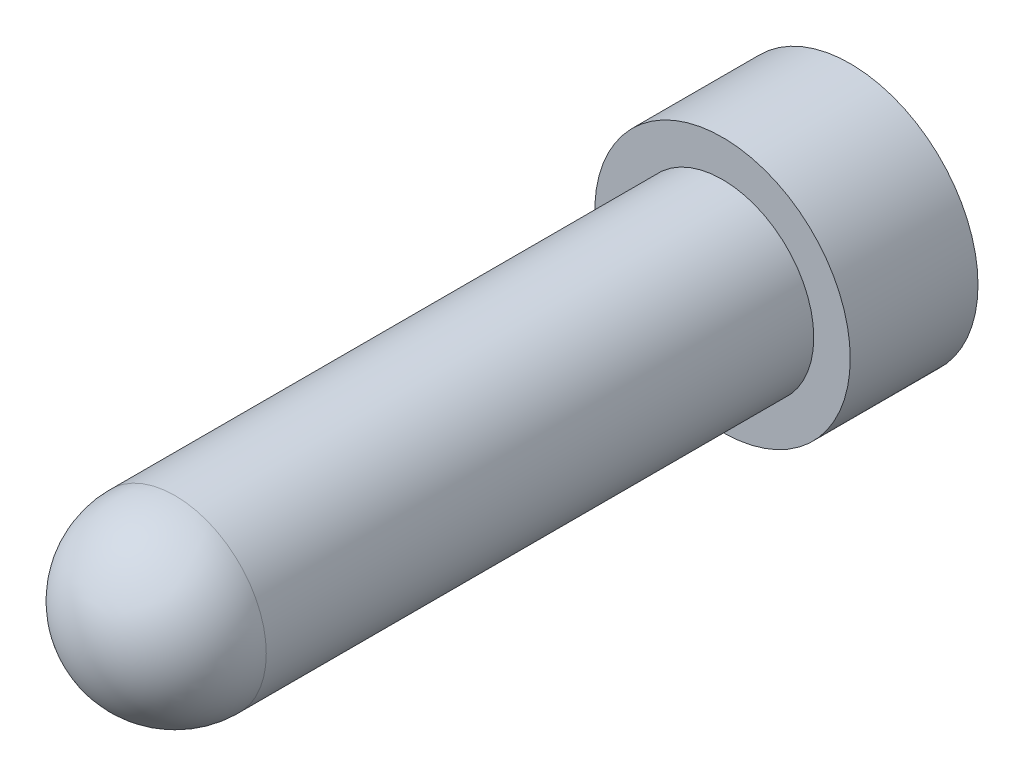
ISO-10303-21;
HEADER;
FILE_DESCRIPTION(('STEP AP214'),'2;1');
FILE_NAME('part.step','',(''),(''),'','','');
FILE_SCHEMA(('AUTOMOTIVE_DESIGN { 1 0 10303 214 1 1 1 1 }'));
ENDSEC;
DATA;
#1=APPLICATION_CONTEXT('core data for automotive mechanical design processes');
#2=APPLICATION_PROTOCOL_DEFINITION('international standard','automotive_design',2000,#1);
#3=PRODUCT_CONTEXT('',#1,'mechanical');
#4=PRODUCT('Part','Part','',(#3));
#5=PRODUCT_RELATED_PRODUCT_CATEGORY('part','',(#4));
#6=PRODUCT_DEFINITION_FORMATION('','',#4);
#7=PRODUCT_DEFINITION_CONTEXT('part definition',#1,'design');
#8=PRODUCT_DEFINITION('design','',#6,#7);
#9=PRODUCT_DEFINITION_SHAPE('','',#8);
#10=(LENGTH_UNIT() NAMED_UNIT(*) SI_UNIT(.MILLI.,.METRE.));
#11=(NAMED_UNIT(*) PLANE_ANGLE_UNIT() SI_UNIT($,.RADIAN.));
#12=(NAMED_UNIT(*) SI_UNIT($,.STERADIAN.) SOLID_ANGLE_UNIT());
#13=UNCERTAINTY_MEASURE_WITH_UNIT(LENGTH_MEASURE(1.E-05),#10,'distance_accuracy_value','');
#14=(GEOMETRIC_REPRESENTATION_CONTEXT(3) GLOBAL_UNCERTAINTY_ASSIGNED_CONTEXT((#13)) GLOBAL_UNIT_ASSIGNED_CONTEXT((#10,
#11,#12)) REPRESENTATION_CONTEXT('',''));
#15=CARTESIAN_POINT('',(0.,0.,0.));
#16=DIRECTION('',(0.,0.,1.));
#17=DIRECTION('',(1.,0.,0.));
#18=AXIS2_PLACEMENT_3D('',#15,#16,#17);
#19=CARTESIAN_POINT('',(0.,0.,7.));
#20=DIRECTION('',(0.,0.,-1.));
#21=DIRECTION('',(-1.,0.,0.));
#22=AXIS2_PLACEMENT_3D('',#19,#20,#21);
#23=CYLINDRICAL_SURFACE('',#22,7.);
#24=CARTESIAN_POINT('',(0.,0.,7.));
#25=DIRECTION('',(0.,0.,1.));
#26=DIRECTION('',(1.,0.,0.));
#27=AXIS2_PLACEMENT_3D('',#24,#25,#26);
#28=CIRCLE('',#27,7.);
#29=CARTESIAN_POINT('',(7.,0.,7.));
#30=VERTEX_POINT('',#29);
#31=EDGE_CURVE('E149',#30,#30,#28,.T.);
#32=ORIENTED_EDGE('',*,*,#31,.F.);
#33=EDGE_LOOP('',(#32));
#34=FACE_BOUND('',#33,.T.);
#35=CARTESIAN_POINT('',(0.,0.,0.));
#36=DIRECTION('',(0.,0.,1.));
#37=DIRECTION('',(1.,0.,0.));
#38=AXIS2_PLACEMENT_3D('',#35,#36,#37);
#39=CIRCLE('',#38,7.);
#40=CARTESIAN_POINT('',(7.,0.,0.));
#41=VERTEX_POINT('',#40);
#42=EDGE_CURVE('E143',#41,#41,#39,.T.);
#43=ORIENTED_EDGE('',*,*,#42,.T.);
#44=EDGE_LOOP('',(#43));
#45=FACE_BOUND('',#44,.T.);
#46=ADVANCED_FACE('F39',(#34,#45),#23,.T.);
#47=CARTESIAN_POINT('',(0.,0.,7.));
#48=DIRECTION('',(0.,0.,1.));
#49=DIRECTION('',(1.,0.,0.));
#50=AXIS2_PLACEMENT_3D('',#47,#48,#49);
#51=PLANE('',#50);
#52=CARTESIAN_POINT('',(0.,0.,7.));
#53=DIRECTION('',(0.,0.,1.));
#54=DIRECTION('',(1.,0.,0.));
#55=AXIS2_PLACEMENT_3D('',#52,#53,#54);
#56=CIRCLE('',#55,5.);
#57=CARTESIAN_POINT('',(5.,0.,7.));
#58=VERTEX_POINT('',#57);
#59=EDGE_CURVE('E50',#58,#58,#56,.T.);
#60=ORIENTED_EDGE('',*,*,#59,.F.);
#61=EDGE_LOOP('',(#60));
#62=FACE_BOUND('',#61,.T.);
#63=ORIENTED_EDGE('',*,*,#31,.T.);
#64=EDGE_LOOP('',(#63));
#65=FACE_BOUND('',#64,.T.);
#66=ADVANCED_FACE('F158',(#62,#65),#51,.T.);
#67=CARTESIAN_POINT('',(0.,0.,0.));
#68=DIRECTION('',(0.,0.,1.));
#69=DIRECTION('',(1.,0.,0.));
#70=AXIS2_PLACEMENT_3D('',#67,#68,#69);
#71=PLANE('',#70);
#72=DIRECTION('',(0.5,0.866025403784439,0.));
#73=VECTOR('',#72,1.);
#74=CARTESIAN_POINT('',(-5.77350269189626,0.,0.));
#75=LINE('',#74,#73);
#76=CARTESIAN_POINT('',(-5.77350269189626,0.,0.));
#77=VERTEX_POINT('',#76);
#78=CARTESIAN_POINT('',(-2.88675134594813,5.,0.));
#79=VERTEX_POINT('',#78);
#80=EDGE_CURVE('E126',#77,#79,#75,.T.);
#81=ORIENTED_EDGE('',*,*,#80,.F.);
#82=DIRECTION('',(-0.5,0.866025403784439,0.));
#83=VECTOR('',#82,1.);
#84=CARTESIAN_POINT('',(-2.88675134594813,-5.,0.));
#85=LINE('',#84,#83);
#86=CARTESIAN_POINT('',(-2.88675134594813,-5.,0.));
#87=VERTEX_POINT('',#86);
#88=EDGE_CURVE('E53',#87,#77,#85,.T.);
#89=ORIENTED_EDGE('',*,*,#88,.F.);
#90=DIRECTION('',(-1.,0.,0.));
#91=VECTOR('',#90,1.);
#92=CARTESIAN_POINT('',(2.88675134594813,-5.,0.));
#93=LINE('',#92,#91);
#94=CARTESIAN_POINT('',(2.88675134594813,-5.,0.));
#95=VERTEX_POINT('',#94);
#96=EDGE_CURVE('E140',#95,#87,#93,.T.);
#97=ORIENTED_EDGE('',*,*,#96,.F.);
#98=DIRECTION('',(-0.5,-0.866025403784439,0.));
#99=VECTOR('',#98,1.);
#100=CARTESIAN_POINT('',(5.77350269189626,0.,0.));
#101=LINE('',#100,#99);
#102=CARTESIAN_POINT('',(5.77350269189626,0.,0.));
#103=VERTEX_POINT('',#102);
#104=EDGE_CURVE('E132',#103,#95,#101,.T.);
#105=ORIENTED_EDGE('',*,*,#104,.F.);
#106=DIRECTION('',(0.5,-0.866025403784439,0.));
#107=VECTOR('',#106,1.);
#108=CARTESIAN_POINT('',(2.88675134594813,5.,0.));
#109=LINE('',#108,#107);
#110=CARTESIAN_POINT('',(2.88675134594813,5.,0.));
#111=VERTEX_POINT('',#110);
#112=EDGE_CURVE('E105',#111,#103,#109,.T.);
#113=ORIENTED_EDGE('',*,*,#112,.F.);
#114=DIRECTION('',(1.,0.,0.));
#115=VECTOR('',#114,1.);
#116=CARTESIAN_POINT('',(-2.88675134594813,5.,0.));
#117=LINE('',#116,#115);
#118=EDGE_CURVE('E133',#79,#111,#117,.T.);
#119=ORIENTED_EDGE('',*,*,#118,.F.);
#120=EDGE_LOOP('',(#81,#89,#97,#105,#113,#119));
#121=FACE_BOUND('',#120,.T.);
#122=ORIENTED_EDGE('',*,*,#42,.F.);
#123=EDGE_LOOP('',(#122));
#124=FACE_BOUND('',#123,.T.);
#125=ADVANCED_FACE('F154',(#121,#124),#71,.F.);
#126=CARTESIAN_POINT('',(0.,0.,42.));
#127=DIRECTION('',(0.,0.,-1.));
#128=DIRECTION('',(-1.,0.,0.));
#129=AXIS2_PLACEMENT_3D('',#126,#127,#128);
#130=CYLINDRICAL_SURFACE('',#129,5.);
#131=CARTESIAN_POINT('',(0.,0.,37.));
#132=DIRECTION('',(0.,0.,-1.));
#133=DIRECTION('',(-1.,0.,0.));
#134=AXIS2_PLACEMENT_3D('',#131,#132,#133);
#135=CIRCLE('',#134,5.);
#136=CARTESIAN_POINT('',(-5.,0.,37.));
#137=VERTEX_POINT('',#136);
#138=EDGE_CURVE('E11',#137,#137,#135,.T.);
#139=ORIENTED_EDGE('',*,*,#138,.T.);
#140=EDGE_LOOP('',(#139));
#141=FACE_BOUND('',#140,.T.);
#142=ORIENTED_EDGE('',*,*,#59,.T.);
#143=EDGE_LOOP('',(#142));
#144=FACE_BOUND('',#143,.T.);
#145=ADVANCED_FACE('F160',(#141,#144),#130,.T.);
#146=CARTESIAN_POINT('',(0.,0.,37.));
#147=DIRECTION('',(0.,0.,1.));
#148=DIRECTION('',(1.,0.,0.));
#149=AXIS2_PLACEMENT_3D('',#146,#147,#148);
#150=SPHERICAL_SURFACE('',#149,5.);
#151=ORIENTED_EDGE('',*,*,#138,.F.);
#152=EDGE_LOOP('',(#151));
#153=FACE_BOUND('',#152,.T.);
#154=ADVANCED_FACE('F41',(#153),#150,.T.);
#155=CARTESIAN_POINT('',(-2.88675134594813,-5.,5.));
#156=DIRECTION('',(-0.866025403784439,-0.5,0.));
#157=DIRECTION('',(0.5,-0.866025403784439,0.));
#158=AXIS2_PLACEMENT_3D('',#155,#156,#157);
#159=PLANE('',#158);
#160=ORIENTED_EDGE('',*,*,#88,.T.);
#161=DIRECTION('',(0.,0.,-1.));
#162=VECTOR('',#161,1.);
#163=CARTESIAN_POINT('',(-5.77350269189626,0.,5.));
#164=LINE('',#163,#162);
#165=CARTESIAN_POINT('',(-5.77350269189626,0.,5.));
#166=VERTEX_POINT('',#165);
#167=EDGE_CURVE('E82',#166,#77,#164,.T.);
#168=ORIENTED_EDGE('',*,*,#167,.F.);
#169=DIRECTION('',(-0.5,0.866025403784439,0.));
#170=VECTOR('',#169,1.);
#171=CARTESIAN_POINT('',(-2.88675134594813,-5.,5.));
#172=LINE('',#171,#170);
#173=CARTESIAN_POINT('',(-2.88675134594813,-5.,5.));
#174=VERTEX_POINT('',#173);
#175=EDGE_CURVE('E137',#174,#166,#172,.T.);
#176=ORIENTED_EDGE('',*,*,#175,.F.);
#177=DIRECTION('',(0.,0.,-1.));
#178=VECTOR('',#177,1.);
#179=CARTESIAN_POINT('',(-2.88675134594813,-5.,5.));
#180=LINE('',#179,#178);
#181=EDGE_CURVE('E65',#174,#87,#180,.T.);
#182=ORIENTED_EDGE('',*,*,#181,.T.);
#183=EDGE_LOOP('',(#160,#168,#176,#182));
#184=FACE_BOUND('',#183,.T.);
#185=ADVANCED_FACE('F193',(#184),#159,.F.);
#186=CARTESIAN_POINT('',(2.88675134594813,-5.,5.));
#187=DIRECTION('',(0.,-1.,0.));
#188=DIRECTION('',(0.,0.,-1.));
#189=AXIS2_PLACEMENT_3D('',#186,#187,#188);
#190=PLANE('',#189);
#191=ORIENTED_EDGE('',*,*,#96,.T.);
#192=ORIENTED_EDGE('',*,*,#181,.F.);
#193=DIRECTION('',(-1.,0.,0.));
#194=VECTOR('',#193,1.);
#195=CARTESIAN_POINT('',(2.88675134594813,-5.,5.));
#196=LINE('',#195,#194);
#197=CARTESIAN_POINT('',(2.88675134594813,-5.,5.));
#198=VERTEX_POINT('',#197);
#199=EDGE_CURVE('E111',#198,#174,#196,.T.);
#200=ORIENTED_EDGE('',*,*,#199,.F.);
#201=DIRECTION('',(0.,0.,-1.));
#202=VECTOR('',#201,1.);
#203=CARTESIAN_POINT('',(2.88675134594813,-5.,5.));
#204=LINE('',#203,#202);
#205=EDGE_CURVE('E106',#198,#95,#204,.T.);
#206=ORIENTED_EDGE('',*,*,#205,.T.);
#207=EDGE_LOOP('',(#191,#192,#200,#206));
#208=FACE_BOUND('',#207,.T.);
#209=ADVANCED_FACE('F204',(#208),#190,.F.);
#210=CARTESIAN_POINT('',(5.77350269189626,0.,5.));
#211=DIRECTION('',(0.866025403784439,-0.5,0.));
#212=DIRECTION('',(0.5,0.866025403784439,0.));
#213=AXIS2_PLACEMENT_3D('',#210,#211,#212);
#214=PLANE('',#213);
#215=ORIENTED_EDGE('',*,*,#104,.T.);
#216=ORIENTED_EDGE('',*,*,#205,.F.);
#217=DIRECTION('',(-0.5,-0.866025403784439,0.));
#218=VECTOR('',#217,1.);
#219=CARTESIAN_POINT('',(5.77350269189626,0.,5.));
#220=LINE('',#219,#218);
#221=CARTESIAN_POINT('',(5.77350269189626,0.,5.));
#222=VERTEX_POINT('',#221);
#223=EDGE_CURVE('E109',#222,#198,#220,.T.);
#224=ORIENTED_EDGE('',*,*,#223,.F.);
#225=DIRECTION('',(0.,0.,-1.));
#226=VECTOR('',#225,1.);
#227=CARTESIAN_POINT('',(5.77350269189626,0.,5.));
#228=LINE('',#227,#226);
#229=EDGE_CURVE('E92',#222,#103,#228,.T.);
#230=ORIENTED_EDGE('',*,*,#229,.T.);
#231=EDGE_LOOP('',(#215,#216,#224,#230));
#232=FACE_BOUND('',#231,.T.);
#233=ADVANCED_FACE('F112',(#232),#214,.F.);
#234=CARTESIAN_POINT('',(2.88675134594813,5.,5.));
#235=DIRECTION('',(0.866025403784439,0.5,0.));
#236=DIRECTION('',(-0.5,0.866025403784439,0.));
#237=AXIS2_PLACEMENT_3D('',#234,#235,#236);
#238=PLANE('',#237);
#239=ORIENTED_EDGE('',*,*,#112,.T.);
#240=ORIENTED_EDGE('',*,*,#229,.F.);
#241=DIRECTION('',(0.5,-0.866025403784439,0.));
#242=VECTOR('',#241,1.);
#243=CARTESIAN_POINT('',(2.88675134594813,5.,5.));
#244=LINE('',#243,#242);
#245=CARTESIAN_POINT('',(2.88675134594813,5.,5.));
#246=VERTEX_POINT('',#245);
#247=EDGE_CURVE('E97',#246,#222,#244,.T.);
#248=ORIENTED_EDGE('',*,*,#247,.F.);
#249=DIRECTION('',(0.,0.,-1.));
#250=VECTOR('',#249,1.);
#251=CARTESIAN_POINT('',(2.88675134594813,5.,5.));
#252=LINE('',#251,#250);
#253=EDGE_CURVE('E110',#246,#111,#252,.T.);
#254=ORIENTED_EDGE('',*,*,#253,.T.);
#255=EDGE_LOOP('',(#239,#240,#248,#254));
#256=FACE_BOUND('',#255,.T.);
#257=ADVANCED_FACE('F100',(#256),#238,.F.);
#258=CARTESIAN_POINT('',(-2.88675134594813,5.,5.));
#259=DIRECTION('',(0.,1.,0.));
#260=DIRECTION('',(-1.,0.,0.));
#261=AXIS2_PLACEMENT_3D('',#258,#259,#260);
#262=PLANE('',#261);
#263=ORIENTED_EDGE('',*,*,#118,.T.);
#264=ORIENTED_EDGE('',*,*,#253,.F.);
#265=DIRECTION('',(1.,0.,0.));
#266=VECTOR('',#265,1.);
#267=CARTESIAN_POINT('',(-2.88675134594813,5.,5.));
#268=LINE('',#267,#266);
#269=CARTESIAN_POINT('',(-2.88675134594813,5.,5.));
#270=VERTEX_POINT('',#269);
#271=EDGE_CURVE('E117',#270,#246,#268,.T.);
#272=ORIENTED_EDGE('',*,*,#271,.F.);
#273=DIRECTION('',(0.,0.,-1.));
#274=VECTOR('',#273,1.);
#275=CARTESIAN_POINT('',(-2.88675134594813,5.,5.));
#276=LINE('',#275,#274);
#277=EDGE_CURVE('E145',#270,#79,#276,.T.);
#278=ORIENTED_EDGE('',*,*,#277,.T.);
#279=EDGE_LOOP('',(#263,#264,#272,#278));
#280=FACE_BOUND('',#279,.T.);
#281=ADVANCED_FACE('F229',(#280),#262,.F.);
#282=CARTESIAN_POINT('',(-5.77350269189626,0.,5.));
#283=DIRECTION('',(-0.866025403784438,0.5,0.));
#284=DIRECTION('',(-0.5,-0.866025403784439,0.));
#285=AXIS2_PLACEMENT_3D('',#282,#283,#284);
#286=PLANE('',#285);
#287=ORIENTED_EDGE('',*,*,#80,.T.);
#288=ORIENTED_EDGE('',*,*,#277,.F.);
#289=DIRECTION('',(0.5,0.866025403784439,0.));
#290=VECTOR('',#289,1.);
#291=CARTESIAN_POINT('',(-5.77350269189626,0.,5.));
#292=LINE('',#291,#290);
#293=EDGE_CURVE('E125',#166,#270,#292,.T.);
#294=ORIENTED_EDGE('',*,*,#293,.F.);
#295=ORIENTED_EDGE('',*,*,#167,.T.);
#296=EDGE_LOOP('',(#287,#288,#294,#295));
#297=FACE_BOUND('',#296,.T.);
#298=ADVANCED_FACE('F236',(#297),#286,.F.);
#299=CARTESIAN_POINT('',(0.,0.,5.));
#300=DIRECTION('',(0.,0.,-1.));
#301=DIRECTION('',(-1.,0.,0.));
#302=AXIS2_PLACEMENT_3D('',#299,#300,#301);
#303=PLANE('',#302);
#304=ORIENTED_EDGE('',*,*,#175,.T.);
#305=ORIENTED_EDGE('',*,*,#293,.T.);
#306=ORIENTED_EDGE('',*,*,#271,.T.);
#307=ORIENTED_EDGE('',*,*,#247,.T.);
#308=ORIENTED_EDGE('',*,*,#223,.T.);
#309=ORIENTED_EDGE('',*,*,#199,.T.);
#310=EDGE_LOOP('',(#304,#305,#306,#307,#308,#309));
#311=FACE_BOUND('',#310,.T.);
#312=ADVANCED_FACE('F120',(#311),#303,.T.);
#313=CLOSED_SHELL('',(#46,#66,#125,#145,#154,#185,#209,#233,#257,#281,#298,#312));
#314=MANIFOLD_SOLID_BREP('B2',#313);
#315=ADVANCED_BREP_SHAPE_REPRESENTATION('',(#18,#314),#14);
#316=SHAPE_DEFINITION_REPRESENTATION(#9,#315);
ENDSEC;
END-ISO-10303-21;
